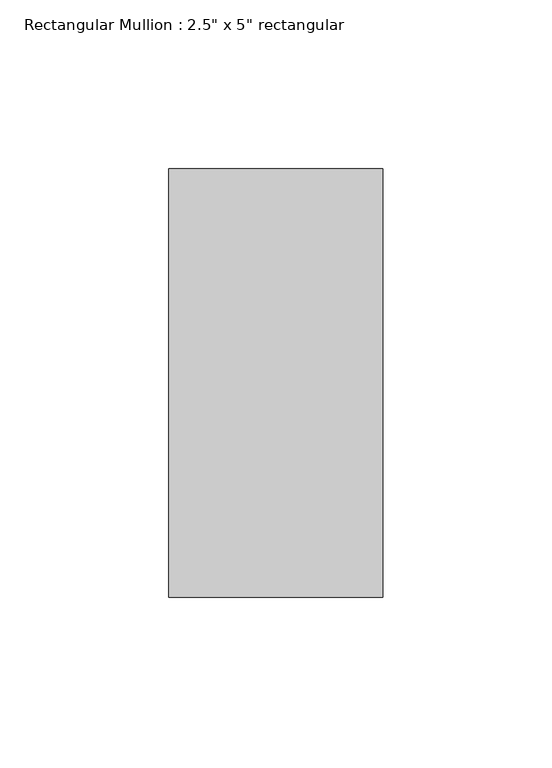
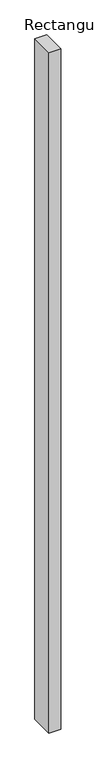
"""IFC4 building model written with IfcOpenShell, lengths in millimetres: member geometry."""

from ifc_helpers import new_model, si_unit, frame, origin, place, context, project, spatial, polyline, outline, extrude, source, transform, mapped, element, save


def member_2115025b(model_context):
    return source(origin(), model_context, "Body", "SweptSolid", [
        extrude(outline(polyline([(0.0, 63.5), (0.0, -63.5), (-63.5, -63.5), (-63.5, 63.5), (0.0, 63.5)])), frame((0.0, 0.0, -3793.3826946), z_axis=(0.0, 0.0, 1.0), x_axis=(1.0, 0.0, 0.0)), (0.0, 0.0, 1.0), 3793.3826946),
    ])


if __name__ == "__main__":
    model = new_model("IFC4")
    model_context = context("Model", 3, world=origin())
    ifc_project = project(units=[si_unit("LENGTHUNIT", "METRE", prefix="MILLI")], contexts=[model_context])
    site = spatial("IfcSite", under=ifc_project)
    building = spatial("IfcBuilding", under=site)
    placement = place(None, origin())
    member_shape = member_2115025b(model_context)
    element("IfcMember", 1, ObjectType="Rectangular Mullion : 2.5\" x 5\" rectangular", at=placement, inside=building, context=model_context, shape_type="MappedRepresentation", body=[
        mapped(member_shape, transform((0.0, 0.0, 0.0), x_axis=(1.0, 0.0, 0.0), y_axis=(0.0, 1.0, 0.0), z_axis=(0.0, 0.0, 1.0))),
    ])
    save(model, "model.ifc")

# Revit data of these elements
# Type "Rectangular Mullion : 2.5\" x 5\" rectangular"
#   built-in parameter 1007304 = 0.416667 (stored number, unit not read)
#   built-in parameter 1007301 = 0.104167 (stored number, unit not read)
#   built-in parameter 1007300 = 0.104167 (stored number, unit not read)
# Element 1 (IfcMember, "Rectangular Mullion : 2.5\" x 5\" rectangular")
#   Materials on its faces: "Iron, Ductile"
# Materials
#   "Iron, Ductile": class "Metal", colour RGB 0 0 0, transparency 0, Description = "Ductile cast iron", Cost = 0
